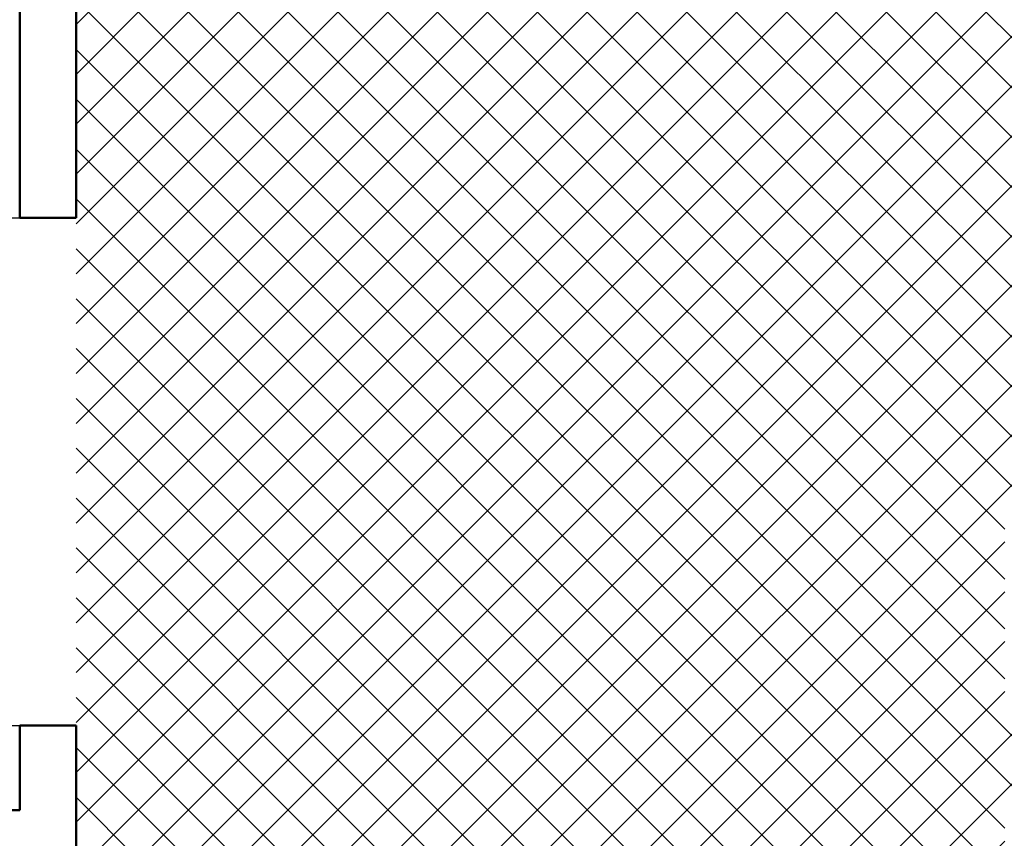
# Model space of a CAD drawing. Units: inches. Extents: x -466983 to 1020, y 324 to 318697.
# Tile 48 of 97: x 609 to 679, y 827 to 885. Entities that reach past the tile are written whole.
import ezdxf

# ---------------------------------------------------------------- set-up
doc = ezdxf.new("R2010")
doc.units = ezdxf.units.IN
doc.header["$MEASUREMENT"] = 0
for name, color, linetype, lineweight in [('A-DOOR', 3, 'Continuous', 25), ('A-FLOR-PATT', 252, 'Continuous', 13), ('A-WALL', 7, 'Continuous', 50)]:
    doc.layers.add(name, color=color, linetype=linetype, lineweight=lineweight)

# ---------------------------------------------------------------- blocks, each defined once
blk = doc.blocks.new('*U33')
for p, q in [((0, 0), (0, -6)), ((40, 0), (40, -6))]:
    blk.add_line(p, q)
blk.add_lwpolyline([(0, 0), (0, 40), (1.75, 40), (1.75, 0)], close=True)
blk.add_arc((0, 0), 40, 0, 90)

msp = doc.modelspace()

# ---------------------------------------------------------------- hatches: boundary and pattern name
at = {"layer": 'A-FLOR-PATT', "transparency": 33554572}
h = msp.add_hatch(dxfattribs=at)
h.set_pattern_fill('ANSI37', color=256, scale=30)
h.set_pattern_definition([(45, (-1212.4137, -290.035), (-2.6516504, 2.6516504), []), (135, (-1212.4137, -290.035), (-2.6516504, -2.6516504), [])])
h.paths.add_polyline_path([(901.806, 1075.938), (900.614, 1075.938), (900.614, 1065.386), (899.391, 1065.386), (898.091, 1065.386), (892.836, 1058.71, -0.258377), (892.188, 1058.351), (879.985, 1058.351, -0.20177), (879.438, 1058.581), (874.081, 1065.386), (872.781, 1065.386), (871.558, 1065.386), (871.558, 1075.938), (813.806, 1075.938), (813.806, 1044.792), (832.395, 1044.792, -0.394795), (848.66, 1028.536), (848.66, 1009.938), (901.806, 1009.938), (901.806, 1015.938), (901.306, 1015.938), (871.306, 1015.938), (871.306, 1017.25), (871.334, 1017.25, -0.401453), (901.306, 1045.938), (901.806, 1045.938)])
edge = h.paths.add_edge_path(flags=16)
edge.add_line((847.773, 1068.949), (847.773, 1073.709))
edge.add_arc((849.227, 1073.709), 1.454, 90, 180, ccw=False)
edge.add_line((849.227, 1075.163), (864.492, 1075.163))
edge.add_arc((864.492, 1073.709), 1.454, 0, 90, ccw=False)
edge.add_line((865.946, 1073.709), (865.946, 1069.004))
edge.add_arc((832.645, 1068.976), 33.301, -20.61234, 0.04725, ccw=False)
edge.add_ellipse((856.859, 1058.48), major_axis=(0, 10.213), ratio=0.685919, start_angle=100.00884, end_angle=259.99116, ccw=False)
edge.add_arc((881.074, 1068.976), 33.301, 180.04725, 200.61234, ccw=False)
h.paths.add_polyline_path([(853.146, 1066.482), (853.146, 1066.453), (853.146, 1066.453, 0.433107), (852.917, 1066.685), (852.917, 1066.453), (853.146, 1066.453), (853.146, 1066.482), (853.088, 1066.612, 0.697939), (852.7, 1066.453), (852.7, 1066.453), (852.7, 1066.482), (852.917, 1067.001), (852.917, 1066.685, -0.396254)], flags=0)
h.paths.add_polyline_path([(861.019, 1066.482), (861.019, 1066.453), (861.019, 1066.453, 0.416404), (860.802, 1066.685), (860.802, 1066.453), (861.019, 1066.453), (861.019, 1066.482), (860.967, 1066.605, 0.713344), (860.573, 1066.453), (860.573, 1066.453), (860.573, 1066.482), (860.802, 1067.001), (860.802, 1066.685, -0.379973)], flags=0)
edge = h.paths.add_edge_path(flags=0)
edge.add_spline(control_points=[(861.13, 1065.785), (861.466, 1065.248), (861.613, 1065.016), (861.983, 1064.374), (862.192, 1063.944), (862.561, 1063.039), (862.721, 1062.563), (862.987, 1061.578), (863.092, 1061.069), (863.245, 1060.031), (863.293, 1059.503), (863.329, 1058.441), (863.318, 1057.908), (863.237, 1056.852), (863.166, 1056.329), (862.97, 1055.308), (862.843, 1054.81), (862.537, 1053.852), (862.357, 1053.393), (861.951, 1052.525), (861.725, 1052.117), (861.233, 1051.362), (860.967, 1051.016), (860.405, 1050.395), (860.108, 1050.12), (859.494, 1049.646), (859.176, 1049.448), (858.528, 1049.13), (858.197, 1049.011), (857.531, 1048.852), (857.196, 1048.812), (856.525, 1048.812), (856.189, 1048.852), (855.524, 1049.01), (855.193, 1049.129), (854.545, 1049.447), (854.227, 1049.645), (853.612, 1050.118), (853.316, 1050.393), (852.753, 1051.014), (852.487, 1051.36), (851.995, 1052.114), (851.769, 1052.523), (851.363, 1053.39), (851.183, 1053.85), (850.877, 1054.807), (850.75, 1055.305), (850.553, 1056.326), (850.483, 1056.849), (850.401, 1057.905), (850.39, 1058.438), (850.426, 1059.5), (850.473, 1060.028), (850.626, 1061.066), (850.732, 1061.575), (850.997, 1062.561), (851.157, 1063.036), (851.525, 1063.942), (851.734, 1064.371), (852.106, 1065.016), (852.254, 1065.25), (852.608, 1065.733)], knot_values=[3.915332, 3.915332, 3.915332, 3.915332, 4.013468, 4.013468, 4.175532, 4.175532, 4.337596, 4.337596, 4.49966, 4.49966, 4.661724, 4.661724, 4.823788, 4.823788, 4.985852, 4.985852, 5.147916, 5.147916, 5.30998, 5.30998, 5.472044, 5.472044, 5.634109, 5.634109, 5.796173, 5.796173, 5.958237, 5.958237, 6.120301, 6.120301, 6.282365, 6.282365, 6.444429, 6.444429, 6.606493, 6.606493, 6.768557, 6.768557, 6.930621, 6.930621, 7.092685, 7.092685, 7.254749, 7.254749, 7.416813, 7.416813, 7.578878, 7.578878, 7.740942, 7.740942, 7.903006, 7.903006, 8.06507, 8.06507, 8.227134, 8.227134, 8.389198, 8.389198, 8.551262, 8.551262, 8.65037, 8.65037, 8.65037, 8.65037], degree=3, periodic=0)
edge.add_line((852.642, 1065.785), (861.13, 1065.785))
edge = h.paths.add_edge_path(flags=0)
edge.add_ellipse((856.85, 1057.743), major_axis=(0, 7.792), ratio=0.687861, start_angle=0, end_angle=360)
h.paths.add_polyline_path([(848.863, 1069.389), (848.863, 1073.96, -0.414214), (849.954, 1075.051), (863.765, 1075.051, -0.414214), (864.856, 1073.96), (864.856, 1069.389, -0.388936), (864.524, 1069.027, -0.043561), (849.195, 1069.027, -0.388936)], flags=0)
h.paths.add_polyline_path([(853.101, 1068.112, -1), (852.677, 1068.112, -1)], flags=0)
edge = h.paths.add_edge_path(flags=0)
edge.add_ellipse((856.859, 1057.338), major_axis=(0, 2.207), ratio=0.657164, start_angle=0, end_angle=360)
h.paths.add_polyline_path([(861.041, 1068.112, -1), (860.618, 1068.112, -1)], flags=0)
edge = h.paths.add_edge_path()
edge.add_line((573.954, 1057.341), (573.954, 1075.938))
edge.add_line((573.954, 1075.938), (558.731, 1075.938))
edge.add_line((558.731, 1075.938), (558.731, 1065.386))
edge.add_line((558.731, 1065.386), (557.507, 1065.386))
edge.add_line((557.507, 1065.386), (556.207, 1065.386))
edge.add_line((556.207, 1065.386), (550.952, 1058.71))
edge.add_arc((550.304, 1059.116), 0.765, 270, 327.94832, ccw=False)
edge.add_line((550.304, 1058.351), (538.101, 1058.351))
edge.add_arc((538.101, 1059.116), 0.765, 224.3704, 270, ccw=False)
edge.add_line((537.555, 1058.581), (532.198, 1065.386))
edge.add_line((532.198, 1065.386), (530.898, 1065.386))
edge.add_line((530.898, 1065.386), (529.674, 1065.386))
edge.add_line((529.674, 1065.386), (529.674, 1075.938))
edge.add_line((529.674, 1075.938), (520.806, 1075.938))
edge.add_line((520.806, 1075.938), (520.806, 1045.938))
edge.add_line((520.806, 1045.938), (521.306, 1045.938))
edge.add_arc((521.306, 1015.938), 30, 2.50749, 90, ccw=False)
edge.add_line((551.277, 1017.25), (551.306, 1017.25))
edge.add_line((551.306, 1017.25), (551.306, 1015.938))
edge.add_line((551.306, 1015.938), (520.806, 1015.938))
edge.add_line((520.806, 1015.938), (520.806, 1009.938))
edge.add_line((520.806, 1009.938), (559.191, 1010.402))
edge.add_arc((559.191, 1011.856), 1.454, 180, 270, ccw=False)
edge.add_line((557.737, 1011.856), (557.737, 1016.561))
edge.add_arc((591.039, 1016.589), 33.301, 159.38766, 180.04725, ccw=False)
edge.add_ellipse((566.824, 1027.085), major_axis=(0, 10.213), ratio=0.685919, start_angle=280.00884, end_angle=439.99116, ccw=False)
edge.add_arc((542.609, 1016.589), 33.301, 0.04725, 20.61234, ccw=False)
edge.add_line((575.91, 1016.616), (575.91, 1011.856))
edge.add_arc((574.456, 1011.856), 1.454, -90, 0, ccw=False)
edge.add_line((574.456, 1010.402), (608.806, 1009.938))
edge.add_line((608.806, 1009.938), (608.806, 1041.086))
edge.add_line((608.806, 1041.086), (590.218, 1041.086))
edge.add_arc((590.775, 1057.907), 16.831, 181.92775, 268.10321, ccw=False)
edge = h.paths.add_edge_path()
edge.add_ellipse((494.244, 583.62), major_axis=(0, 10.213), ratio=0.685919, start_angle=280.00884, end_angle=439.99116, ccw=False)
edge.add_arc((470.03, 573.124), 33.301, 0.04725, 20.61234, ccw=False)
edge.add_line((503.331, 573.152), (503.331, 568.392))
edge.add_arc((501.877, 568.392), 1.454, -90, 0, ccw=False)
edge.add_line((501.877, 566.938), (539.806, 566.938))
edge.add_line((539.806, 566.938), (539.806, 572.938))
edge.add_line((539.806, 572.938), (539.306, 572.938))
edge.add_line((539.306, 572.938), (509.306, 572.938))
edge.add_line((509.306, 572.938), (509.306, 574.25))
edge.add_line((509.306, 574.25), (509.334, 574.25))
edge.add_arc((539.306, 572.938), 30, 90, 177.49251, ccw=False)
edge.add_line((539.306, 602.938), (539.806, 602.938))
edge.add_line((539.806, 602.938), (539.806, 626.938))
edge.add_line((539.806, 626.938), (531.772, 626.938))
edge.add_line((531.772, 626.938), (531.772, 616.386))
edge.add_line((531.772, 616.386), (530.548, 616.386))
edge.add_line((530.548, 616.386), (529.249, 616.386))
edge.add_line((529.249, 616.386), (523.711, 609.351))
edge.add_line((523.711, 609.351), (510.777, 609.351))
edge.add_line((510.777, 609.351), (505.239, 616.386))
edge.add_line((505.239, 616.386), (503.939, 616.386))
edge.add_line((503.939, 616.386), (502.715, 616.386))
edge.add_line((502.715, 616.386), (502.715, 626.938))
edge.add_line((502.715, 626.938), (481.698, 626.938))
edge.add_line((481.698, 626.938), (481.698, 610.995))
edge.add_arc((467.27, 611.473), 14.436, 271.92775, 358.10321, ccw=False)
edge.add_line((467.756, 597.045), (451.806, 597.045))
edge.add_line((451.806, 597.045), (451.806, 584.404))
edge.add_line((451.806, 584.404), (451.806, 566.938))
edge.add_line((451.806, 566.938), (486.612, 566.938))
edge.add_arc((486.612, 568.392), 1.454, 180, 270, ccw=False)
edge.add_line((485.158, 568.392), (485.158, 573.097))
edge.add_arc((518.459, 573.124), 33.301, 159.38766, 180.04725, ccw=False)
h.paths.add_polyline_path([(836.261, 1020.733), (879.89, 1020.733), (879.89, 1039.39), (836.261, 1039.39)], flags=25)
h.paths.add_polyline_path([(549.985, 1036.749), (593.614, 1036.749), (593.614, 1055.407), (549.985, 1055.407)], flags=24)
h.paths.add_polyline_path([(475.123, 595.596), (518.752, 595.596), (518.752, 614.253), (475.123, 614.253)], flags=24)
h = msp.add_hatch(dxfattribs=at)
h.set_pattern_fill('ANSI37', color=256, scale=20)
h.set_pattern_definition([(45, (-1212.4137, -290.035), (-1.767767, 1.767767), []), (135, (-1212.4137, -290.035), (-1.767767, -1.767767), [])])
h.paths.add_polyline_path([(809.806, 870.938), (809.806, 888.152), (806.998, 888.152), (802.662, 888.152), (789.383, 888.152), (786.285, 888.152, -0.414214), (785.499, 888.937), (785.499, 900.196), (785.499, 908.47, -0.414214), (786.808, 909.779, -0.414214), (785.499, 911.088), (785.499, 929.101, -0.414214), (786.808, 930.411, -0.414214), (785.499, 931.72), (785.499, 931.904, -0.414214), (784.19, 930.595), (766.722, 930.595, -0.412359), (765.413, 931.896, -0.413741), (764.115, 930.578), (744.578, 930.422, -0.416556), (743.786, 931.207), (743.786, 933.515), (742.215, 933.515), (742.215, 952.024, -0.001344), (743.786, 952.2), (743.786, 953.938), (678.592, 953.938), (678.592, 951.131), (678.592, 946.794), (678.592, 933.515), (678.592, 930.417, -0.414214), (677.806, 929.631), (666.548, 929.631), (658.274, 929.631, -0.414214), (656.965, 930.94, -0.414214), (655.656, 929.631), (637.642, 929.631, -0.414214), (636.333, 930.94, -0.414214), (635.024, 929.631), (634.839, 929.631, -0.414214), (636.149, 928.322), (636.149, 910.854, -0.412359), (634.848, 909.545, -0.413741), (636.165, 908.247), (636.321, 888.71, -0.416556), (635.536, 887.918), (633.228, 887.918), (633.228, 886.347), (614.719, 886.347, -0.001344), (614.544, 887.918), (612.806, 887.918), (612.806, 834.938), (612.806, 752.938), (612.806, 748.938), (612.806, 697.938), (654.806, 697.938), (654.806, 701.938), (715.806, 701.938), (715.806, 737.435), (774.292, 737.435), (774.292, 795.938), (809.806, 795.938)])
h.paths.add_polyline_path([(679.276, 849.576, 0.102523), (682.148, 849.261, -0.080461), (694.543, 849.773, -0.283899), (694.482, 849.008, 0.136605), (694.407, 848.81, -0.030441), (694.543, 846.893), (694.543, 842.62), (694.543, 838.347, -0.028219), (694.425, 836.568), (694.425, 836.568, 0.196187), (694.446, 836.271, -0.302897), (694.543, 835.467, -0.080461), (682.148, 835.979, 0.102523), (679.276, 835.664, -0.58611), (678.646, 836.017), (678.646, 849.223, -0.58611)], flags=16)
h.paths.add_polyline_path([(679.517, 848.651, 0.699597), (679.476, 848.634, 1.20716), (679.194, 848.742, 0.010621)], flags=0)
h.paths.add_polyline_path([(679.492, 836.561, -0.013798), (679.918, 836.659, -0.071703), (682.853, 837.143, -0.165743), (682.166, 839.101), (682.166, 842.609), (682.166, 846.06, -0.240616), (683.473, 848.677, -0.068263), (693.929, 849.008), (693.788, 848.708), (693.788, 849.023, 0.067332), (683.473, 848.677, 0.240616), (682.166, 846.06), (682.166, 842.609), (682.166, 839.101, 0.23459), (683.461, 836.551, 0.068093), (693.788, 836.195), (693.788, 836.51), (693.93, 836.21, -0.077215), (682.242, 836.782, 0.086627), (679.528, 836.57, -0.628402), (679.503, 836.573), (679.503, 836.607, 0.910458)], flags=0)
h.paths.add_polyline_path([(679.476, 848.636), (679.207, 848.647), (679.207, 836.572, 0.913566), (679.365, 836.586), (679.476, 836.582)], flags=0)
h.paths.add_polyline_path([(679.276, 829.86, 0.102523), (682.148, 829.546, -0.080461), (694.543, 830.057, -0.283899), (694.482, 829.293, 0.136605), (694.407, 829.095, -0.030441), (694.543, 827.178), (694.543, 822.904), (694.543, 818.631, -0.028219), (694.425, 816.853), (694.425, 816.853, 0.196187), (694.446, 816.556, -0.302897), (694.543, 815.752, -0.080461), (682.148, 816.263, 0.102523), (679.276, 815.949, -0.58611), (678.646, 816.302), (678.646, 829.507, -0.58611)], flags=16)
h.paths.add_polyline_path([(679.517, 828.936, 0.699597), (679.476, 828.919, 1.20716), (679.194, 829.027, 0.010621)], flags=0)
h.paths.add_polyline_path([(679.492, 816.846, -0.013798), (679.918, 816.944, -0.071703), (682.853, 817.428, -0.165743), (682.166, 819.385), (682.166, 822.894), (682.166, 826.345, -0.240616), (683.473, 828.961, -0.068263), (693.929, 829.293), (693.788, 828.993), (693.788, 829.308, 0.067332), (683.473, 828.961, 0.240616), (682.166, 826.345), (682.166, 822.894), (682.166, 819.385, 0.23459), (683.461, 816.836, 0.068093), (693.788, 816.48), (693.788, 816.795), (693.93, 816.495, -0.077215), (682.242, 817.066, 0.086627), (679.528, 816.855, -0.628402), (679.503, 816.858), (679.503, 816.892, 0.910458)], flags=0)
h.paths.add_polyline_path([(679.476, 828.921), (679.207, 828.932), (679.207, 816.857, 0.913566), (679.365, 816.871), (679.476, 816.867)], flags=0)
h.paths.add_polyline_path([(679.276, 810.145, 0.102523), (682.148, 809.83, -0.080461), (694.543, 810.342, -0.3023), (694.447, 809.539, 0.10023), (694.406, 809.388, -0.03057), (694.543, 807.462), (694.543, 803.189), (694.543, 798.916, -0.03057), (694.406, 796.991, 0.10023), (694.447, 796.839, -0.3023), (694.543, 796.036, -0.080461), (682.148, 796.548, 0.102523), (679.276, 796.233, -0.58611), (678.646, 796.586), (678.646, 809.792, -0.58611)], flags=16)
h.paths.add_polyline_path([(679.517, 809.242, 0.699597), (679.476, 809.224, 1.20716), (679.194, 809.332, 0.010621)], flags=0)
h.paths.add_polyline_path([(679.492, 797.151, -0.013798), (679.918, 797.25, -0.071703), (682.853, 797.734, -0.165743), (682.166, 799.691), (682.166, 803.2), (682.166, 806.65, -0.239349), (683.461, 809.258, -0.072465), (694.447, 809.541, 0.197932), (694.425, 809.241), (693.788, 809.299), (693.788, 809.614, 0.068093), (683.461, 809.258, 0.239349), (682.166, 806.65), (682.166, 803.2), (682.166, 799.691, 0.235854), (683.473, 797.132, 0.067332), (693.788, 796.786), (693.788, 797.101), (694.425, 797.159, 0.197932), (694.447, 796.859, -0.080419), (682.156, 797.379, 0.083867), (679.528, 797.16, -0.628402), (679.503, 797.164), (679.503, 797.197, 0.910458)], flags=0)
h.paths.add_polyline_path([(679.207, 809.237), (679.207, 797.162, 0.913566), (679.365, 797.176), (679.476, 797.173), (679.476, 809.227)], flags=0)
h.paths.add_polyline_path([(695.364, 853.299), (728.223, 853.299), (728.223, 771.152), (695.364, 771.152)], flags=16)
h.paths.add_polyline_path([(696.021, 852.642), (727.566, 852.642), (727.566, 771.809), (696.021, 771.809)], flags=0)
h.paths.add_polyline_path([(679.276, 788.787, 0.102523), (682.148, 788.472, -0.080461), (694.543, 788.984, -0.3023), (694.447, 788.181, 0.10023), (694.406, 788.03, -0.03057), (694.543, 786.104), (694.543, 781.831), (694.543, 777.558, -0.03057), (694.406, 775.632, 0.10023), (694.447, 775.481, -0.3023), (694.543, 774.678, -0.080461), (682.148, 775.19, 0.102523), (679.276, 774.875, -0.58611), (678.646, 775.228), (678.646, 788.434, -0.58611)], flags=16)
h.paths.add_polyline_path([(679.517, 787.883, 0.699597), (679.476, 787.866, 1.20716), (679.194, 787.974, 0.010621)], flags=0)
h.paths.add_polyline_path([(679.492, 775.793, -0.013798), (679.918, 775.891, -0.071703), (682.853, 776.375, -0.165743), (682.166, 778.333), (682.166, 781.841), (682.166, 785.292, -0.239349), (683.461, 787.899, -0.072465), (694.447, 788.182, 0.197932), (694.425, 787.882), (693.788, 787.94), (693.788, 788.255, 0.068093), (683.461, 787.899, 0.239349), (682.166, 785.292), (682.166, 781.841), (682.166, 778.333, 0.235854), (683.473, 775.774, 0.067332), (693.788, 775.428), (693.788, 775.742), (694.425, 775.8, 0.197932), (694.447, 775.5, -0.080419), (682.156, 776.021, 0.083867), (679.528, 775.802, -0.628402), (679.503, 775.805), (679.503, 775.839, 0.910458)], flags=0)
h.paths.add_polyline_path([(679.207, 787.879), (679.207, 775.804, 0.913566), (679.365, 775.818), (679.476, 775.814), (679.476, 787.868)], flags=0)
h.paths.add_polyline_path([(704.641, 854.12, -0.080461), (705.153, 866.516, 0.102523), (704.838, 869.387, -0.58611), (705.191, 870.017), (718.397, 870.017, -0.58611), (718.75, 869.387, 0.102523), (718.435, 866.516, -0.080461), (718.946, 854.12, -0.3023), (718.144, 854.217, 0.10023), (717.992, 854.257, -0.03057), (716.067, 854.12), (711.794, 854.12), (707.521, 854.12, -0.03057), (705.595, 854.257, 0.10023), (705.444, 854.217, -0.3023)], flags=16)
h.paths.add_polyline_path([(717.846, 869.146, 0.699597), (717.829, 869.187, 1.20716), (717.937, 869.47, 0.010621)], flags=0)
h.paths.add_polyline_path([(705.463, 854.216, -0.080419), (705.984, 866.507, 0.083867), (705.765, 869.135, -0.628402), (705.768, 869.16), (705.802, 869.16, 0.910458), (705.756, 869.171, -0.013798), (705.854, 868.745, -0.071703), (706.338, 865.81, -0.165743), (708.295, 866.497), (711.804, 866.497), (715.255, 866.497, -0.239349), (717.862, 865.202, -0.072465), (718.145, 854.216, 0.197932), (717.845, 854.238), (717.903, 854.876), (718.218, 854.876, 0.068093), (717.862, 865.202, 0.239349), (715.255, 866.497), (711.804, 866.497), (708.295, 866.497, 0.235854), (705.737, 865.19, 0.067332), (705.391, 854.876), (705.705, 854.876), (705.763, 854.238, 0.197932)], flags=16)
h.paths.add_polyline_path([(705.766, 869.456, 0.913566), (705.781, 869.299), (705.777, 869.187), (717.831, 869.187), (717.842, 869.456)], flags=0)
h.paths.add_polyline_path([(729.045, 842.62), (729.045, 846.893, -0.03057), (729.182, 848.818, 0.10023), (729.141, 848.97, -0.3023), (729.045, 849.773, -0.080461), (741.44, 849.261, 0.102523), (744.311, 849.576, -0.58611), (744.942, 849.223), (744.942, 836.017, -0.58611), (744.311, 835.664, 0.102523), (741.44, 835.979, -0.080461), (729.045, 835.467, -0.3023), (729.141, 836.27, 0.10023), (729.182, 836.421, -0.03057), (729.045, 838.347)], flags=16)
h.paths.add_polyline_path([(744.111, 836.585, 1.20716), (744.394, 836.477, 0.010621), (744.07, 836.567, 0.699597)], flags=0)
h.paths.add_polyline_path([(729.141, 836.268, 0.197932), (729.162, 836.568), (729.8, 836.51), (729.8, 836.195, 0.068093), (740.126, 836.551, 0.239349), (741.421, 839.159), (741.421, 842.609), (741.421, 846.118, 0.235854), (740.114, 848.677, 0.067332), (729.8, 849.023), (729.8, 848.708), (729.162, 848.65, 0.197932), (729.141, 848.95, -0.080419), (741.432, 848.43, 0.083867), (744.059, 848.649, -0.628402), (744.085, 848.645), (744.085, 848.612, 0.910458), (744.095, 848.658, -0.013798), (743.67, 848.559, -0.071703), (740.734, 848.075, -0.165743), (741.421, 846.118), (741.421, 842.609), (741.421, 839.159, -0.239349), (740.126, 836.551, -0.072465)], flags=0)
h.paths.add_polyline_path([(729.045, 830.057, -0.080461), (741.44, 829.546, 0.102523), (744.311, 829.86, -0.58611), (744.942, 829.507), (744.942, 816.302, -0.58611), (744.311, 815.949, 0.102523), (741.44, 816.263, -0.080461), (729.045, 815.752, -0.3023), (729.141, 816.554, 0.10023), (729.182, 816.706, -0.03057), (729.045, 818.631), (729.045, 822.904), (729.045, 827.178, -0.03057), (729.182, 829.103, 0.10023), (729.141, 829.255, -0.3023)], flags=16)
h.paths.add_polyline_path([(744.111, 816.869, 1.20716), (744.394, 816.761, 0.010621), (744.07, 816.852, 0.699597)], flags=0)
h.paths.add_polyline_path([(729.141, 829.235, -0.080419), (741.432, 828.714, 0.083867), (744.059, 828.933, -0.628402), (744.085, 828.93), (744.085, 828.896, 0.910458), (744.095, 828.943, -0.013798), (743.67, 828.844, -0.071703), (740.734, 828.36, -0.165743), (741.421, 826.403), (741.421, 822.894), (741.421, 819.443, -0.239349), (740.126, 816.836, -0.072465), (729.141, 816.553, 0.197932), (729.162, 816.853), (729.8, 816.795), (729.8, 816.48, 0.068093), (740.126, 816.836, 0.239349), (741.421, 819.443), (741.421, 822.894), (741.421, 826.403, 0.235854), (740.114, 828.961, 0.067332), (729.8, 829.308), (729.8, 828.993), (729.162, 828.935, 0.197932)], flags=16)
h.paths.add_polyline_path([(729.045, 810.342, -0.080461), (741.44, 809.83, 0.102523), (744.311, 810.145, -0.58611), (744.942, 809.792), (744.942, 796.586, -0.58611), (744.311, 796.233, 0.102523), (741.44, 796.548, -0.080461), (729.045, 796.036, -0.283899), (729.105, 796.801, 0.136605), (729.181, 796.999, -0.030441), (729.045, 798.916), (729.045, 803.189), (729.045, 807.462, -0.028219), (729.163, 809.241), (729.162, 809.241, 0.196187), (729.142, 809.538, -0.302897)], flags=16)
h.paths.add_polyline_path([(744.111, 797.175, 1.20716), (744.394, 797.067, 0.010621), (744.07, 797.158, 0.699597)], flags=0)
h.paths.add_polyline_path([(741.345, 809.027, 0.086627), (744.059, 809.239, -0.628402), (744.085, 809.235), (744.085, 809.202, 0.910458), (744.095, 809.248, -0.013798), (743.67, 809.15, -0.071703), (740.734, 808.666, -0.165743), (741.421, 806.708), (741.421, 803.2), (741.421, 799.749, -0.240616), (740.114, 797.132, -0.068263), (729.658, 796.801), (729.8, 797.101), (729.8, 796.786, 0.067332), (740.114, 797.132, 0.240616), (741.421, 799.749), (741.421, 803.2), (741.421, 806.708, 0.23459), (740.126, 809.258, 0.068093), (729.8, 809.614), (729.8, 809.299), (729.658, 809.599, -0.077215)], flags=0)
h.paths.add_polyline_path([(704.641, 770.33, -0.283899), (705.405, 770.27, 0.136605), (705.603, 770.194, -0.030441), (707.521, 770.33), (711.794, 770.33), (716.067, 770.33, -0.028219), (717.845, 770.212), (717.845, 770.213, 0.196187), (718.143, 770.233, -0.302897), (718.946, 770.33, -0.080461), (718.435, 757.935, 0.102523), (718.75, 755.064, -0.58611), (718.397, 754.433), (705.191, 754.433, -0.58611), (704.838, 755.064, 0.102523), (705.153, 757.935, -0.080461)], flags=16)
h.paths.add_polyline_path([(705.762, 755.305, 0.699597), (705.779, 755.264, 1.20716), (705.671, 754.981, 0.010621)], flags=0)
h.paths.add_polyline_path([(705.405, 769.717), (705.705, 769.575), (705.391, 769.575, 0.067332), (705.737, 759.261, 0.240616), (708.353, 757.954), (711.804, 757.954), (715.313, 757.954, 0.23459), (717.862, 759.249, 0.068093), (718.218, 769.575), (717.903, 769.575), (718.203, 769.717, -0.077215), (717.632, 758.03, 0.086627), (717.843, 755.316, -0.628402), (717.84, 755.29), (717.806, 755.29, 0.910458), (717.853, 755.28, -0.013798), (717.754, 755.705, -0.071703), (717.27, 758.641, -0.165743), (715.313, 757.954), (711.804, 757.954), (708.353, 757.954, -0.240616), (705.737, 759.261, -0.068263)], flags=0)
h.paths.add_polyline_path([(729.045, 788.984, -0.080461), (741.44, 788.472, 0.102523), (744.311, 788.787, -0.58611), (744.942, 788.434), (744.942, 775.228, -0.58611), (744.311, 774.875, 0.102523), (741.44, 775.19, -0.080461), (729.045, 774.678, -0.283899), (729.105, 775.443, 0.136605), (729.181, 775.64, -0.030441), (729.045, 777.558), (729.045, 781.831), (729.045, 786.104, -0.028219), (729.163, 787.882), (729.162, 787.882, 0.196187), (729.142, 788.18, -0.302897)], flags=16)
h.paths.add_polyline_path([(744.111, 775.817, 1.20716), (744.394, 775.709, 0.010621), (744.07, 775.799, 0.699597)], flags=0)
h.paths.add_polyline_path([(741.345, 787.669, 0.086627), (744.059, 787.881, -0.628402), (744.085, 787.877), (744.085, 787.844, 0.910458), (744.095, 787.89, -0.013798), (743.67, 787.791, -0.071703), (740.734, 787.307, -0.165743), (741.421, 785.35), (741.421, 781.841), (741.421, 778.39, -0.240616), (740.114, 775.774, -0.068263), (729.658, 775.443), (729.8, 775.742), (729.8, 775.428, 0.067332), (740.114, 775.774, 0.240616), (741.421, 778.39), (741.421, 781.841), (741.421, 785.35, 0.23459), (740.126, 787.899, 0.068093), (729.8, 788.255), (729.8, 787.94), (729.658, 788.241, -0.077215)], flags=0)
h.paths.add_polyline_path([(744.111, 848.636), (744.111, 836.582), (744.381, 836.572), (744.381, 848.647, 0.913566), (744.223, 848.633)], flags=0)
h.paths.add_polyline_path([(744.223, 828.917), (744.111, 828.921), (744.111, 816.867), (744.381, 816.857), (744.381, 828.932, 0.913566)], flags=0)
h.paths.add_polyline_path([(717.831, 755.264), (705.777, 755.264), (705.766, 754.994), (717.842, 754.994, 0.913566), (717.827, 755.152)], flags=0)
h.paths.add_polyline_path([(744.223, 809.223), (744.111, 809.227), (744.111, 797.173), (744.381, 797.162), (744.381, 809.237, 0.913566)], flags=0)
h.paths.add_polyline_path([(744.111, 787.868), (744.111, 775.814), (744.381, 775.804), (744.381, 787.879, 0.913566), (744.223, 787.865)], flags=0)
h.paths.add_polyline_path([(678.877, 877.123), (737.613, 877.123), (737.613, 899.512), (678.877, 899.512)], flags=24)

# ---------------------------------------------------------------- linework, layer by layer
at = {"layer": 'A-WALL'}
for p, q in [((608.806, 870.938), (608.806, 1005.938)), ((612.806, 870.938), (612.806, 953.938)), ((612.806, 870.938), (608.806, 870.938)), ((612.806, 834.938), (608.806, 834.938)), ((608.806, 828.938), (608.806, 834.938)), ((612.806, 752.938), (612.806, 834.938)), ((608.806, 828.938), (451.806, 828.938))]:
    msp.add_line(p, q, dxfattribs=at)

# ---------------------------------------------------------------- block references
at = {"layer": 'A-DOOR', "xscale": 0.9000000000000004, "yscale": 0.9000000000000004, "zscale": 0.9000000000000004, "rotation": 90}
msp.add_blockref('*U33', (607.406, 834.938), dxfattribs=at)

doc.saveas('drawing.dxf')
